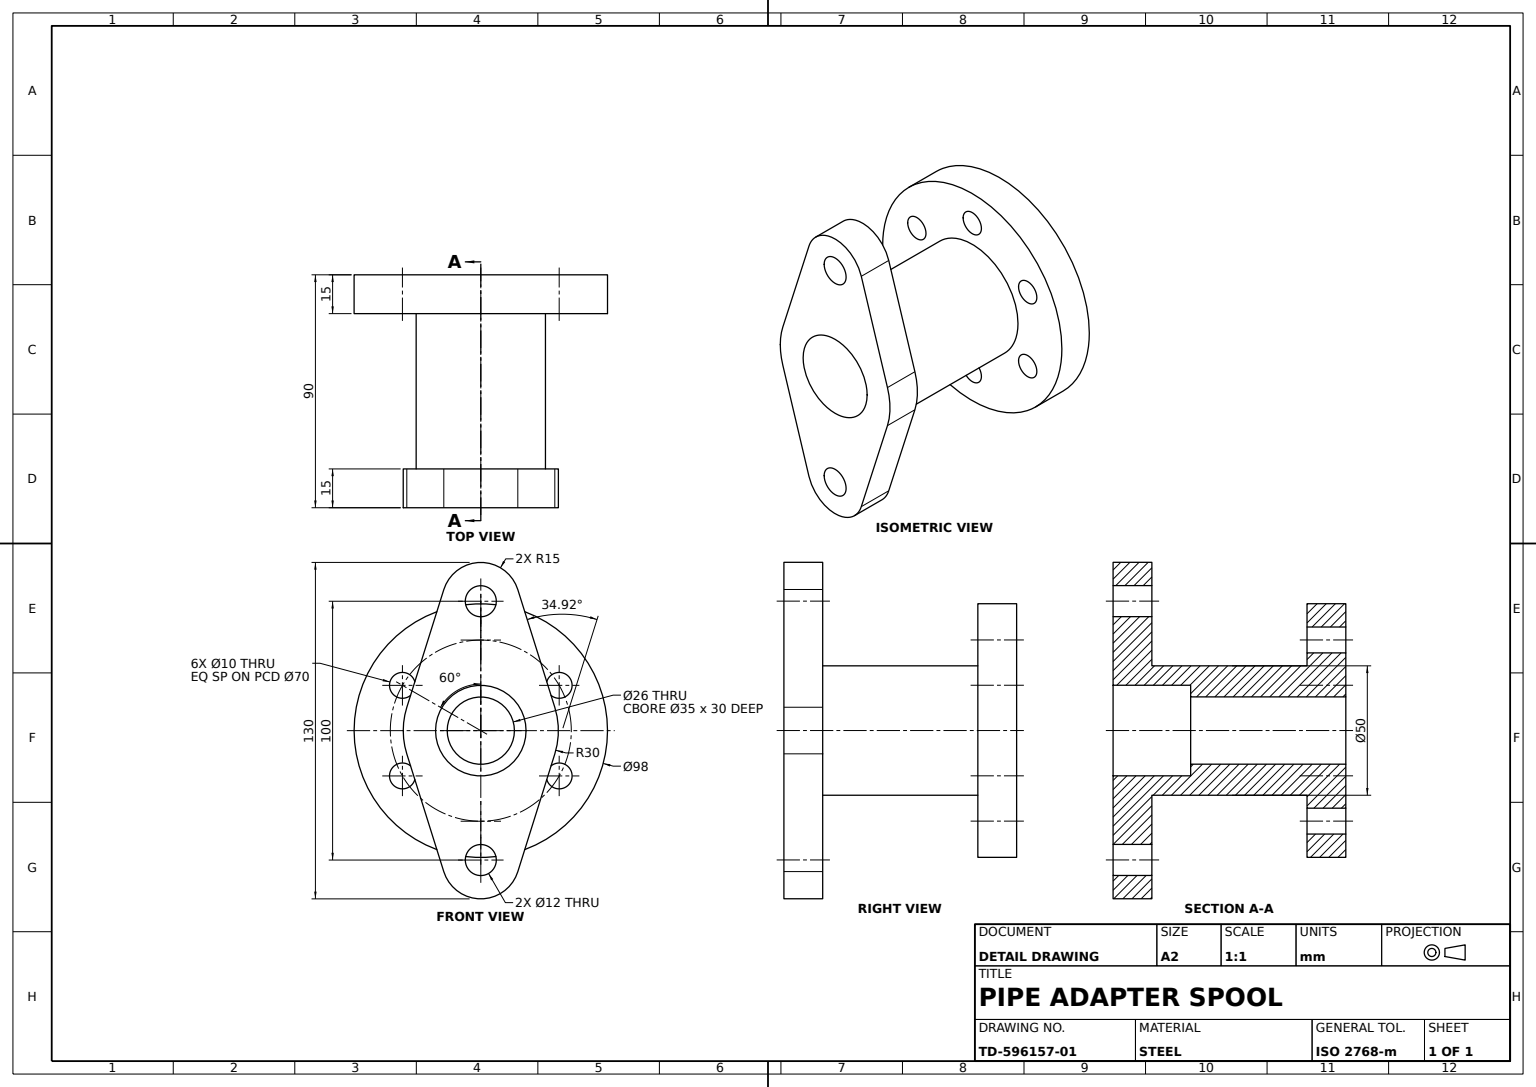
from build123d import *

# Parameters (mm, degrees)
ROUND_FLANGE_SKETCH_R       = 49
ROUND_FLANGE_SKETCH_R_2     = 13
ROUND_FLANGE_SKETCH_R_3     = 5
ROUND_FLANGE_98_6X_10_DEPTH = 15
TUBE_SKETCH_R               = 25
TUBE_SKETCH_R_2             = 13
TUBE_50_BORE_26_DEPTH       = 45
COLLAR_SKETCH_R             = 25
COLLAR_SKETCH_R_2           = 17.5
COLLAR_DEPTH                = 15
OVAL_FLANGE_SKETCH_R        = 25
OVAL_FLANGE_SKETCH_R_2      = 17.5
OVAL_FLANGE_SKETCH_R_3      = 15
OVAL_FLANGE_SKETCH_R_4      = 6
OVAL_FLANGE_2X_12_DEPTH     = 15


with BuildPart() as part:
    # Round Flange Sketch → Round Flange Ø98 6xØ10 (new body)
    with BuildSketch(Plane.XY):
        Circle(ROUND_FLANGE_SKETCH_R)
        Circle(ROUND_FLANGE_SKETCH_R_2, mode=Mode.SUBTRACT)
        with Locations((0, 35)):
            Circle(ROUND_FLANGE_SKETCH_R_3, mode=Mode.SUBTRACT)
        with Locations((30.310889132, 17.5)):
            Circle(ROUND_FLANGE_SKETCH_R_3, mode=Mode.SUBTRACT)
        with Locations((30.310889132, -17.5)):
            Circle(ROUND_FLANGE_SKETCH_R_3, mode=Mode.SUBTRACT)
        with Locations((0, -35)):
            Circle(ROUND_FLANGE_SKETCH_R_3, mode=Mode.SUBTRACT)
        with Locations((-30.310889132, -17.5)):
            Circle(ROUND_FLANGE_SKETCH_R_3, mode=Mode.SUBTRACT)
        with Locations((-30.310889132, 17.5)):
            Circle(ROUND_FLANGE_SKETCH_R_3, mode=Mode.SUBTRACT)
    extrude(amount=ROUND_FLANGE_98_6X_10_DEPTH)

    # Tube Sketch → Tube Ø50 Bore Ø26 (add)
    with BuildSketch(Plane.XY.offset(15)):
        with Locations(Location((0, 0, 0), (0, 0, 180))):
            Circle(TUBE_SKETCH_R)
        Circle(TUBE_SKETCH_R_2, mode=Mode.SUBTRACT)
    extrude(amount=TUBE_50_BORE_26_DEPTH)

    # Collar Sketch → Collar (add)
    with BuildSketch(Plane.XY.offset(60)):
        with Locations(Location((0, 0, 0), (0, 0, 180))):
            Circle(COLLAR_SKETCH_R)
        Circle(COLLAR_SKETCH_R_2, mode=Mode.SUBTRACT)
    extrude(amount=COLLAR_DEPTH)

    # Oval Flange Sketch → Oval Flange 2xØ12 (add)
    # profile 1 of 4: a face of its own
    with BuildSketch(Plane.XY.offset(75)):
        with BuildLine():
            Line((-14.309088021, 54.5), (-28.618176043, 9))
            ThreePointArc((-28.618176043, 9), (-30, 0), (-28.618176043, -9))
            Line((-28.618176043, -9), (-14.309088021, -54.5))
            ThreePointArc((-14.309088021, -54.5), (-2.276365489, -35.173734113), (15, -50))
            ThreePointArc((15, -50), (14.826265887, -52.276365489), (14.309088021, -54.5))
            Line((14.309088021, -54.5), (28.618176043, -9))
            ThreePointArc((28.618176043, -9), (30, 0), (28.618176043, 9))
            Line((28.618176043, 9), (14.309088021, 54.5))
            ThreePointArc((14.309088021, 54.5), (14.826265887, 52.276365489), (15, 50))
            ThreePointArc((15, 50), (-2.276365489, 35.173734113), (-14.309088021, 54.5))
        make_face()
        with Locations(Location((0, 0, 0), (0, 0, 180))):
            Circle(OVAL_FLANGE_SKETCH_R, mode=Mode.SUBTRACT)
    # profile 2 of 4: a face of its own
    with BuildSketch(Plane.XY.offset(75)):
        with Locations(Location((0, 0, 0), (0, 0, 180))):
            Circle(OVAL_FLANGE_SKETCH_R)
        Circle(OVAL_FLANGE_SKETCH_R_2, mode=Mode.SUBTRACT)
    # profile 3 of 4: a face of its own
    with BuildSketch(Plane.XY.offset(75)):
        with Locations((0, 50)):
            Circle(OVAL_FLANGE_SKETCH_R_3)
        with Locations((0, 50)):
            Circle(OVAL_FLANGE_SKETCH_R_4, mode=Mode.SUBTRACT)
    # profile 4 of 4: a face of its own
    with BuildSketch(Plane.XY.offset(75)):
        with Locations((0, -50)):
            Circle(OVAL_FLANGE_SKETCH_R_3)
        with Locations((0, -50)):
            Circle(OVAL_FLANGE_SKETCH_R_4, mode=Mode.SUBTRACT)
    extrude(amount=OVAL_FLANGE_2X_12_DEPTH)


solid = part.part
